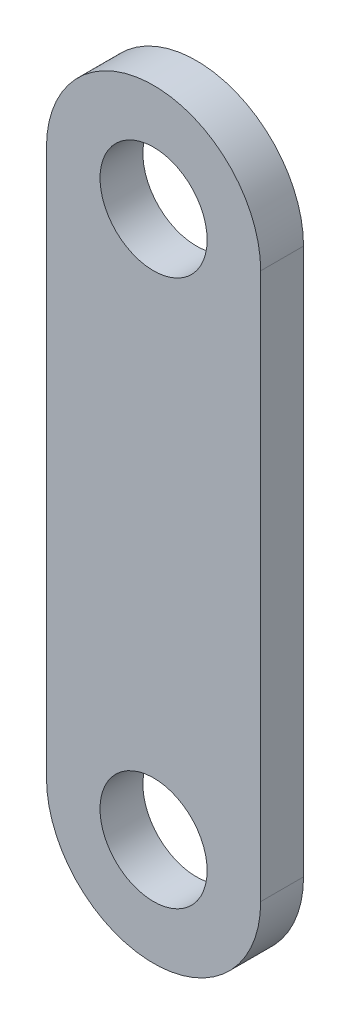
SolidWorks part; units mm, degrees
material "Plain Carbon Steel"
ref_plane "Front Plane" through (0, 0, 0) normal (0, 0, 1) x (1, 0, 0)
ref_plane "Top Plane" through (0, 0, 0) normal (0, 1, 0) x (1, 0, 0)
ref_plane "Right Plane" through (0, 0, 0) normal (1, 0, 0) x (0, 0, -1)
sketch "Link Bar Profile" plane through (0, 0, 0) normal (0, 0, 1) x (1, 0, 0)
  line L0 (0, 0) -> (0, 255) construction
  line L1 (-50, 0) -> (-50, 255)
  line L2 (50, 0) -> (50, 255)
  arc A0 (-50, 0) -> (50, 0) centre (0, 0) ccw
  arc A1 (50, 255) -> (-50, 255) centre (0, 255) ccw
  circle A2 centre (0, 255) radius 25
  circle A3 centre (0, 0) radius 25
  point P3 (0, 127.5)
  dimension "D2" = 50
  dimension "D3" = 25
  dimension "D4" = 25
  dimension "D1" = 255
extrude "Link Bar 20mm" add sketch "Link Bar Profile" along normal blind 20
